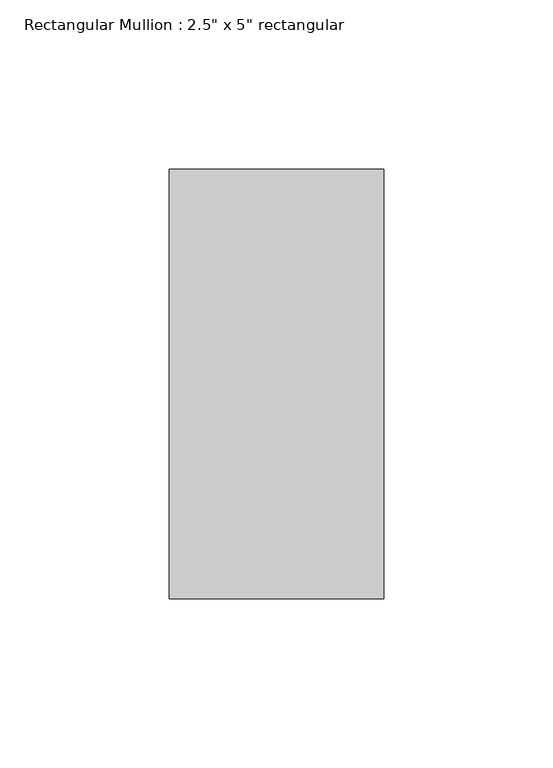
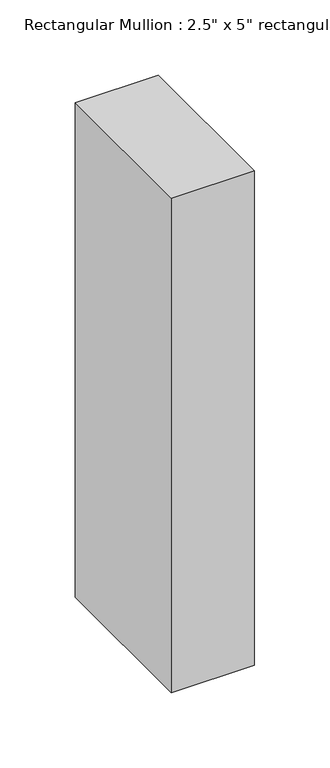
"""IFC4 building model written with IfcOpenShell, lengths in millimetres: member geometry."""

from ifc_helpers import new_model, si_unit, frame, origin, place, context, project, spatial, polyline, outline, extrude, source, transform, mapped, element, save


def member_1ad5418d(model_context):
    return source(origin(), model_context, "Body", "SweptSolid", [
        extrude(outline(polyline([(0.0, 63.5), (0.0, -63.5), (-63.5, -63.5), (-63.5, 63.5), (0.0, 63.5)])), frame((0.0, 0.0, -400.05), z_axis=(0.0, 0.0, 1.0), x_axis=(1.0, 0.0, 0.0)), (0.0, 0.0, 1.0), 400.05),
    ])


if __name__ == "__main__":
    model = new_model("IFC4")
    model_context = context("Model", 3, world=origin())
    ifc_project = project(units=[si_unit("LENGTHUNIT", "METRE", prefix="MILLI")], contexts=[model_context])
    site = spatial("IfcSite", under=ifc_project)
    building = spatial("IfcBuilding", under=site)
    placement = place(None, origin())
    member_shape = member_1ad5418d(model_context)
    element("IfcMember", 1, ObjectType="Rectangular Mullion : 2.5\" x 5\" rectangular", at=placement, inside=building, context=model_context, shape_type="MappedRepresentation", body=[
        mapped(member_shape, transform((0.0, 0.0, 0.0), x_axis=(1.0, 0.0, 0.0), y_axis=(0.0, 1.0, 0.0), z_axis=(0.0, 0.0, 1.0))),
    ])
    save(model, "model.ifc")

# Revit data of these elements
# Type "Rectangular Mullion : 2.5\" x 5\" rectangular"
#   built-in parameter 1007304 = 0.416667 (stored number, unit not read)
#   built-in parameter 1007301 = 0.104167 (stored number, unit not read)
#   built-in parameter 1007300 = 0.104167 (stored number, unit not read)
